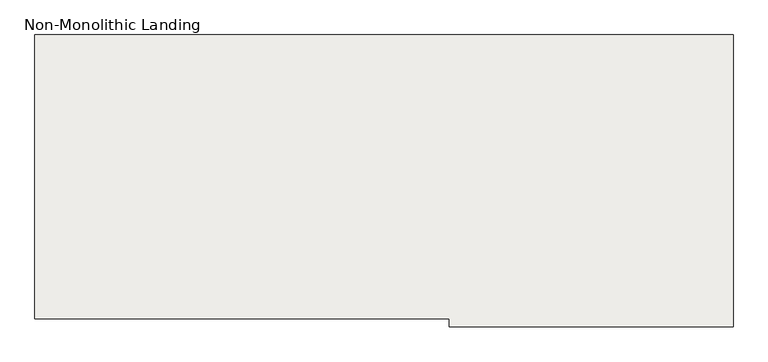
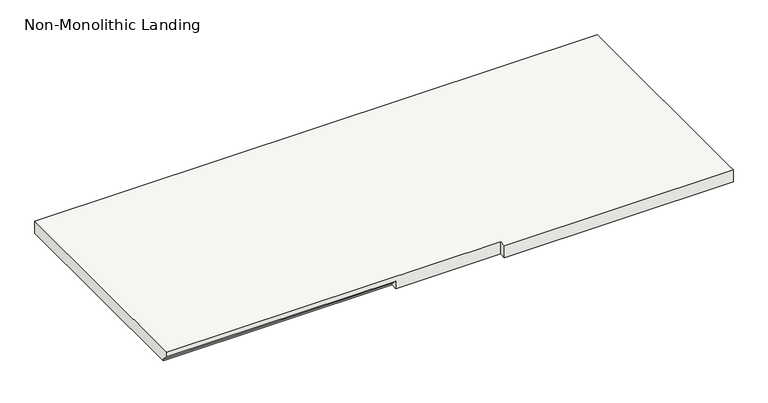
"""IFC4 building model written with IfcOpenShell, lengths in millimetres: slab geometry, Non-Monolithic Landing."""

from ifc_helpers import new_model, si_unit, origin, place, context, project, spatial, faceted_brep, source, transform, mapped, element, save


def non_monolithic_landing_85b13ac5(model_context):
    return source(origin(), model_context, "Body", "Brep", [
        faceted_brep([(131.9501403, 2113.4257925, 5213.35), (131.9501403, 2138.8257925, 5187.95), (1046.3501403, 2138.8257925, 5187.95), (1046.3501403, 2113.4257925, 5213.35), (1465.4501403, 2113.4257925, 5232.4), (1465.4501403, 2088.0257925, 5232.4), (2379.8501403, 2088.0257925, 5232.4), (2379.8501403, 2113.4257925, 5232.4), (2379.8501403, 3027.8257925, 5232.4), (131.9501403, 3027.8257925, 5232.4), (131.9501403, 2113.4257925, 5232.4), (1046.3501403, 2138.8257925, 5181.6), (131.9501403, 2138.8257925, 5181.6), (131.9501403, 3027.8257925, 5181.6), (2379.8501403, 3027.8257925, 5181.6), (2379.8501403, 2113.4257925, 5181.6), (2379.8501403, 2088.0257925, 5181.6), (1465.4501403, 2088.0257925, 5181.6), (1465.4501403, 2113.4257925, 5181.6), (1046.3501403, 2113.4257925, 5181.6)], [[[0, 1, 2, 3]], [[4, 5, 6, 7, 8, 9, 10]], [[11, 12, 13, 14, 15, 16, 17, 18, 19]], [[12, 11, 2, 1]], [[11, 19, 3, 2]], [[4, 10, 0, 3, 19, 18]], [[5, 4, 18, 17]], [[6, 5, 17, 16]], [[7, 6, 16, 15]], [[8, 7, 15, 14]], [[9, 8, 14, 13]], [[10, 9, 13, 12, 1, 0]]]),
    ])


if __name__ == "__main__":
    model = new_model("IFC4")
    model_context = context("Model", 3, world=origin())
    ifc_project = project(units=[si_unit("LENGTHUNIT", "METRE", prefix="MILLI")], contexts=[model_context])
    site = spatial("IfcSite", under=ifc_project)
    building = spatial("IfcBuilding", under=site)
    placement = place(None, origin())
    non_monolithic_landing_shape = non_monolithic_landing_85b13ac5(model_context)
    element("IfcSlab", 1, ObjectType="Non-Monolithic Landing", at=placement, inside=building, context=model_context, shape_type="MappedRepresentation", body=[
        mapped(non_monolithic_landing_shape, transform((0.0, 0.0, 0.0), x_axis=(1.0, 0.0, 0.0), y_axis=(0.0, 1.0, 0.0), z_axis=(0.0, 0.0, 1.0))),
    ])
    save(model, "model.ifc")
